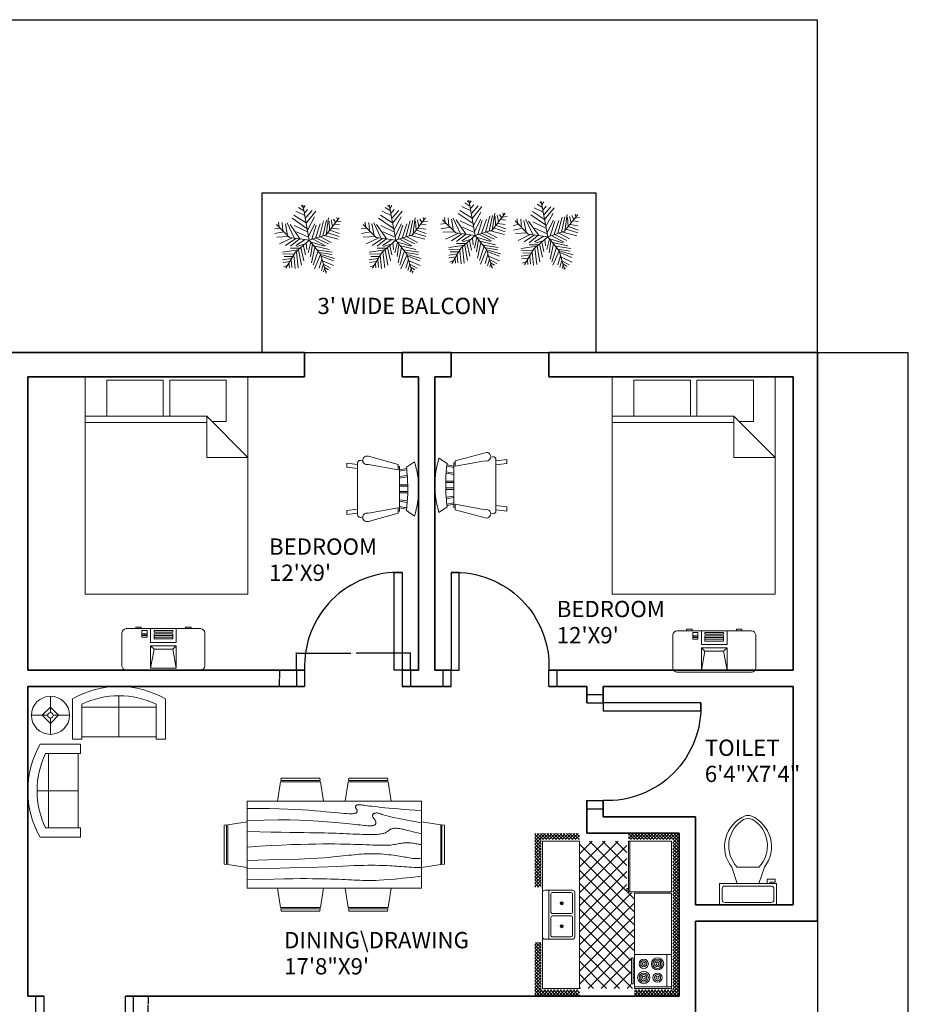
# Model space of a CAD drawing. Units: inches. Extents: x 4159 to 4826, y 299 to 1026.
# Tile 37 of 37: x 4498 to 4826, y 663 to 1026. Entities that reach past the tile are written whole.
import ezdxf

# ---------------------------------------------------------------- set-up
doc = ezdxf.new("R2010")
doc.units = ezdxf.units.IN
for name, color, linetype, lineweight in [('A-ANNO-DIMS', 2, 'Continuous', 18), ('A-AREA-IDEN', 7, 'Continuous', 18), ('A-DOOR', 4, 'Continuous', 25), ('A-EQPM', 8, 'Continuous', 13), ('A-FLOR-BALC', 7, 'Continuous', 25), ('A-FLOR-FIXT', 9, 'Continuous', 18), ('A-FURN', 8, 'Continuous', 18), ('A-WALL', 7, 'Continuous', 35), ('L-PLNT', 94, 'Continuous', 13)]:
    doc.layers.add(name, color=color, linetype=linetype, lineweight=lineweight)
doc.styles.get("Standard").update_dxf_attribs({"font": 'arial.ttf'})
doc.dimstyles.get("Standard").update_dxf_attribs({"dimtxt": 0.18, "dimasz": 0.18, "dimexe": 0.18, "dimexo": 0.0625, "dimgap": 0.09, "dimtad": 0, "dimtih": 1, "dimtoh": 1, "dimdec": 4, "dimzin": 0, "dimdsep": 46, "dimtxsty": 'Standard', "dimcen": 0.09, "dimadec": 0, "dimazin": 0, "dimtfac": 1, "dimtdec": 4, "dimtofl": 0, "dimtmove": 0, "dimatfit": 3, "dimfxl": 1, "dimtolj": 1, "dimtzin": 0, "dimarcsym": 0})

# ---------------------------------------------------------------- blocks, each defined once
blk = doc.blocks.new('Lamp - Table')
for p, q in [((0, 7), (0, 1)), ((-1, 0), (-7, 0)), ((0, 3), (-3, 0)), ((-3, 0), (0, -3)), ((3, 0), (0, 3)), ((0, -3), (3, 0)), ((1, 0), (7, 0)), ((0, -1), (0, -7))]:
    blk.add_line(p, q)
for radius in [7, 1]:
    blk.add_circle((0, 0), radius)
blk = doc.blocks.new('Bed - Queen')
for p, q in [((0, -80.00003), (0, 0)), ((0, 0), (59.99999, 0)), ((59.99999, 0), (59.99999, -80.00003)), ((7.99999, -1.2), (28.79998, -1.2)), ((7.99999, -14.4), (7.99999, -1.2)), ((28.79998, -1.2), (28.79998, -14.4)), ((31.19999, -1.2), (51.99999, -1.2)), ((31.19999, -14.4), (31.19999, -1.2)), ((51.99999, -1.2), (51.99999, -16.4)), ((0, -14.4), (44.8, -14.4)), ((59.99999, -29.6), (44.8, -14.4)), ((44.8, -14.4), (44.8, -29.6)), ((44.8, -16.8), (0, -16.8)), ((51.99999, -16.4), (46.79936, -16.4)), ((44.8, -29.6), (59.99999, -29.6)), ((59.99999, -80.00003), (0, -80.00003))]:
    blk.add_line(p, q)
blk = doc.blocks.new('Chair - Rocking')
for p, q in [((-8, -4.5), (-10, -1.5)), ((8, -4.5), (10, -1.5)), ((-8.23428, -6.99939), (-8.3093, -7.47958)), ((-8.23041, -7), (8.23915, -7)), ((-7.5, -4.5), (-7, -7)), ((-6.5, -7), (-7.02225, -4.43)), ((-4.5, -7), (-4.96674, -4.19951)), ((-4, -7), (-4.40532, -4.16272)), ((-1.5, -4.05012), (-1.5, -7)), ((-1, -7), (-1, -4.05012)), ((1, -7), (1, -4.04655)), ((1.5, -4.05012), (1.5, -7)), ((4, -7), (4.40187, -4.18694)), ((4.5, -7), (4.96761, -4.19437)), ((6.5, -7), (7, -4.4057)), ((7.5, -4.5), (7, -7)), ((8.31071, -7.48854), (8.23449, -7.00073)), ((-9, -7.5), (-12, -18.49999)), ((-7, -7.5), (-9, -7.5)), ((-9, -18.49999), (-7, -7.5)), ((7, -7.5), (9, -7.5)), ((9, -18.49999), (7, -7.5)), ((9, -7.5), (12, -18.49999)), ((-10.36644, -20.64523), (-10.5, -21.49999)), ((10.5, -21.49999), (10.3575, -20.58798)), ((-9, -22.49999), (-9.5, -26.49999)), ((0, -22.49999), (-9.5, -22.49999)), ((-8, -26.49999), (-7.5, -22.49999)), ((0, -22.49999), (9.5, -22.49999)), ((8, -26.49999), (7.5, -22.49999)), ((9, -22.49999), (9.5, -26.49999)), ((-9.5, -26.49999), (-8, -26.49999)), ((9.5, -26.49999), (8, -26.49999))]:
    blk.add_line(p, q)
for centre, radius, start, end in [((0, -34.08333), 34.08333, 72.93847, 107.0615), ((0, -68.25004), 64.25, 93.92211, 97.15267), ((0, -68.25004), 64.25, 82.84733, 93.92211), ((-10.5, -18.99999), 1.58114, 161.5651, 18.43495), ((-9.5, -21.49999), 1, 180, 270), ((10.5, -18.99999), 1.58114, 161.5651, 18.43495), ((9.5, -21.49999), 1, 270, 0)]:
    blk.add_arc(centre, radius, start, end)
blk = doc.blocks.new('Sofa - Roundback Loveseat 5 ft.')
for p, q in [((0, -32.44198), (0, -5.99998)), ((-24, -33.99998), (-24, -11.46958)), ((24.00004, -33.99998), (24.00004, -11.46958)), ((-23.9998, -13.38178), (23.99986, -13.38178)), ((-24, -32.44198), (24.00004, -32.44198))]:
    blk.add_line(p, q)
for points in [[(-24, -33.99998), (-30, -33.99998), (-30, -7.99998)], [(30.00004, -7.99998), (30.00004, -33.99998), (24.00004, -33.99998)]]:
    blk.add_lwpolyline(points)
for centre, radius, start, end in [((0, -60.24998), 60.24998, 60.13715, 119.8628), ((0, -61.38438), 55.38444, 64.32083, 115.6792)]:
    blk.add_arc(centre, radius, start, end)
blk = doc.blocks.new('Dining Set - 36 x 72 in.')
for p, q in [((-22.2343, 26.00059), (-23.4847, 17.99762)), ((-22.2304, 26), (-5.7608, 26)), ((-22, 27.5), (-22.1562, 26.50042)), ((-5.8416, 26.5), (-22.1534, 26.5)), ((-22, 27.5), (-6, 27.5)), ((-5.8437, 26.49966), (-6, 27.5)), ((-4.5152, 17.99762), (-5.7655, 25.99926)), ((5.7657, 26.00059), (4.5153, 17.99762)), ((5.7696, 26), (22.2392, 26)), ((6, 27.5), (5.8438, 26.50042)), ((22.1584, 26.5), (5.8466, 26.5)), ((6, 27.5), (22, 27.5)), ((22.1563, 26.49966), (22, 27.5)), ((23.4848, 17.99762), (22.2345, 25.99926)), ((36, 18), (-36, 18)), ((-36, 18), (-36, -18)), ((36, -18), (36, 18)), ((-45.5, 8), (-44.5004, 8.15617)), ((-44.5, -8.15843), (-44.5, 8.15338)), ((-44.0006, 8.23428), (-35.9976, 9.48474)), ((-44, 8.23041), (-44, -8.23915)), ((44.0006, 8.23428), (35.9976, 9.48474)), ((44, 8.23041), (44, -8.23915)), ((44.5, -8.15843), (44.5, 8.15338)), ((45.5, 8), (44.5005, 8.15617)), ((-45.5, 8), (-45.5, -8)), ((45.5, 8), (45.5, -8)), ((-44.4997, -8.15631), (-45.5, -8)), ((44.4997, -8.15631), (45.5, -8)), ((-35.9976, -9.48476), (-43.9993, -8.2345)), ((35.9976, -9.48476), (43.9993, -8.2345)), ((-36, -18), (36, -18)), ((-22.2343, -26.0006), (-23.4847, -17.99762)), ((-4.5152, -17.99762), (-5.7655, -25.99928)), ((5.7657, -26.0006), (4.5153, -17.99762)), ((23.4848, -17.99762), (22.2345, -25.99928)), ((-22.2304, -26), (-5.7608, -26)), ((-22, -27.5), (-22.1562, -26.50044)), ((-5.8416, -26.5), (-22.1534, -26.5)), ((-22, -27.5), (-6, -27.5)), ((-5.8437, -26.49967), (-6, -27.5)), ((5.7696, -26), (22.2392, -26)), ((6, -27.5), (5.8438, -26.50044)), ((22.1584, -26.5), (5.8466, -26.5)), ((6, -27.5), (22, -27.5)), ((22.1563, -26.49967), (22, -27.5))]:
    blk.add_line(p, q)
for points in [[(-36, 15), (-31.1772, 14.97754), (-26.8079, 14.91406), (-22.8538, 14.81543), (-19.276, 14.6875), (-16.0362, 14.53613), (-13.0957, 14.36718), (-10.4159, 14.18652), (-7.9583, 14), (-5.6904, 13.81315), (-3.6035, 13.63021), (-1.6954, 13.45508), (0.0365, 13.29166), (1.5945, 13.14388), (2.9811, 13.01562), (4.1988, 12.9108), (5.25, 12.83333), (6.1393, 12.78613), (6.8802, 12.76823), (7.4883, 12.77767), (7.9792, 12.8125), (8.3685, 12.87077), (8.6719, 12.95052), (8.9049, 13.0498), (9.0833, 13.16666), (9.2205, 13.29899), (9.3216, 13.44401), (9.3895, 13.59879), (9.4271, 13.76041), (9.4373, 13.92594), (9.4232, 14.09245), (9.3875, 14.257), (9.3333, 14.41666), (9.2638, 14.56917), (9.1836, 14.71484), (9.0975, 14.85465), (9.0104, 14.98958), (8.9272, 15.1206), (8.8529, 15.2487), (8.7922, 15.37483), (8.75, 15.5), (8.7305, 15.62467), (8.7344, 15.74739), (8.7617, 15.86621), (8.8125, 15.97916), (8.8867, 16.08431), (8.9844, 16.17968), (9.1055, 16.26334), (9.25, 16.33333), (9.4189, 16.38802), (9.6172, 16.42708), (9.8506, 16.45052), (10.125, 16.45833), (10.4463, 16.45052), (10.8203, 16.42708), (11.2529, 16.38802), (11.75, 16.33333), (12.3184, 16.26318), (12.9694, 16.17838), (13.7151, 16.07991), (14.5677, 15.96875), (15.5395, 15.84586), (16.6426, 15.71224), (17.8893, 15.56884), (19.2917, 15.41666), (20.859, 15.25667), (22.5879, 15.08984), (24.4721, 14.91715), (26.5052, 14.73958), (28.6809, 14.5581), (30.9929, 14.3737), (33.4347, 14.18733), (36, 14)], [(-36, 10), (-28.9766, 10.14274), (-23.1725, 10.20442), (-18.4241, 10.19775), (-14.5677, 10.13541), (-11.4399, 10.03011), (-8.877, 9.89453), (-6.7154, 9.74137), (-4.7917, 9.58333), (-2.9698, 9.43082), (-1.2246, 9.28515), (0.4415, 9.14534), (2.026, 9.01041), (3.5266, 8.87939), (4.9408, 8.7513), (6.266, 8.62516), (7.5, 8.5), (8.6411, 8.37549), (9.6914, 8.2539), (10.6538, 8.13818), (11.5312, 8.03125), (12.3267, 7.93603), (13.043, 7.85547), (13.6831, 7.79248), (14.25, 7.75), (14.7471, 7.7303), (15.1797, 7.73307), (15.5537, 7.75732), (15.875, 7.80208), (16.1494, 7.86637), (16.3828, 7.94922), (16.5811, 8.04964), (16.75, 8.16666), (16.8944, 8.29915), (17.0143, 8.44531), (17.1089, 8.60319), (17.1771, 8.77083), (17.218, 8.94629), (17.2305, 9.1276), (17.2137, 9.31282), (17.1667, 9.5), (17.0895, 9.6875), (16.987, 9.875), (16.8649, 10.0625), (16.7292, 10.25), (16.5856, 10.4375), (16.4401, 10.625), (16.2985, 10.8125), (16.1667, 11), (16.05, 11.18733), (15.9518, 11.3737), (15.8752, 11.5581), (15.8229, 11.73958), (15.798, 11.91715), (15.8034, 12.08984), (15.842, 12.25667), (15.9167, 12.41666), (16.0295, 12.56836), (16.1784, 12.70833), (16.3605, 12.83268), (16.5729, 12.9375), (16.8127, 13.01888), (17.0768, 13.07291), (17.3625, 13.0957), (17.6667, 13.08333), (17.9894, 13.03312), (18.3418, 12.94726), (18.7382, 12.82918), (19.1927, 12.68229), (19.7195, 12.51001), (20.3327, 12.31575), (21.0465, 12.10294), (21.875, 11.875), (22.8357, 11.63354), (23.959, 11.37304), (25.2786, 11.08618), (26.8282, 10.76562), (28.6414, 10.40405), (30.752, 9.99414), (33.1936, 9.52856), (36, 9)], [(-36, 5.5), (-30.7157, 5.3348), (-26.069, 5.20963), (-21.9946, 5.11767), (-18.4271, 5.05208), (-15.3009, 5.00602), (-12.5508, 4.97265), (-10.1112, 4.94515), (-7.9167, 4.91666), (-5.909, 4.88167), (-4.0586, 4.83984), (-2.3429, 4.79215), (-0.7396, 4.73958), (0.7739, 4.6831), (2.22, 4.6237), (3.6213, 4.56233), (5, 4.5), (6.373, 4.43782), (7.7344, 4.3776), (9.0723, 4.32129), (10.375, 4.27083), (11.6309, 4.22819), (12.8281, 4.19531), (13.9551, 4.17415), (15, 4.16666), (15.954, 4.17448), (16.819, 4.19791), (17.6001, 4.23698), (18.3021, 4.29166), (18.9299, 4.36198), (19.4883, 4.44791), (19.9823, 4.54948), (20.4167, 4.66666), (20.7969, 4.79899), (21.1302, 4.94401), (21.4245, 5.09879), (21.6875, 5.26041), (21.9271, 5.42594), (22.1511, 5.59245), (22.3672, 5.757), (22.5834, 5.91666), (22.8065, 6.06868), (23.0404, 6.21093), (23.2879, 6.34147), (23.5521, 6.45833), (23.8358, 6.55957), (24.142, 6.64323), (24.4735, 6.70735), (24.8334, 6.75), (25.2235, 6.76969), (25.642, 6.76692), (26.0858, 6.74267), (26.5521, 6.69791), (27.0379, 6.63362), (27.5404, 6.55078), (28.0565, 6.45036), (28.5834, 6.33333), (29.1242, 6.19987), (29.7071, 6.04687), (30.3661, 5.87044), (31.1354, 5.66666), (32.0493, 5.43164), (33.142, 5.16146), (34.4475, 4.85221), (36, 4.5)], [(-36, -1), (-30.7915, -0.6591), (-26.0195, -0.38216), (-21.6519, -0.16284), (-17.6563, 0.00521), (-14.0005, 0.12833), (-10.6523, 0.21289), (-7.5796, 0.26522), (-4.75, 0.29166), (-2.134, 0.29793), (0.2878, 0.28711), (2.5317, 0.26163), (4.6146, 0.22396), (6.5529, 0.17651), (8.3633, 0.12174), (10.0623, 0.06209), (11.6667, 0), (13.1899, -0.06201), (14.6341, -0.1211), (15.9982, -0.17432), (17.2813, -0.21875), (18.4823, -0.25147), (19.6003, -0.26953), (20.6343, -0.27002), (21.5834, -0.25), (22.4481, -0.20768), (23.2357, -0.14584), (23.9549, -0.06836), (24.6146, 0.02083), (25.2235, 0.11784), (25.7904, 0.21875), (26.3241, 0.31966), (26.8334, 0.41666), (27.3265, 0.50618), (27.8099, 0.58593), (28.2894, 0.65397), (28.7709, 0.70833), (29.2601, 0.74707), (29.763, 0.76823), (30.2855, 0.76985), (30.8334, 0.75), (31.4088, 0.70784), (31.9994, 0.64713), (32.589, 0.57275), (33.1615, 0.48958), (33.7008, 0.4025), (34.1908, 0.3164), (34.6153, 0.23616), (34.9584, 0.16666), (35.2099, 0.11165), (35.3848, 0.07031), (35.504, 0.04069), (35.5886, 0.02083), (35.6594, 0.00879), (35.7377, 0.0026), (35.8442, 0.00032), (36, 0)], [(-36, -6.5), (-27.1843, -6.31267), (-20.084, -6.1263), (-14.469, -5.9419), (-10.1094, -5.76042), (-6.7752, -5.58285), (-4.2363, -5.41016), (-2.2629, -5.24333), (-0.625, -5.08334), (0.8708, -4.93099), (2.2715, -4.78646), (3.5872, -4.64974), (4.8281, -4.52084), (6.0046, -4.39974), (7.127, -4.28646), (8.2053, -4.18099), (9.25, -4.08334), (10.2705, -3.99382), (11.2734, -3.91407), (12.2647, -3.84603), (13.25, -3.79167), (14.2354, -3.75293), (15.2266, -3.73177), (16.2295, -3.73015), (17.25, -3.75), (18.2912, -3.79248), (19.3451, -3.85547), (20.4009, -3.93604), (21.4479, -4.03125), (22.4754, -4.13819), (23.4727, -4.25391), (24.4289, -4.37549), (25.3334, -4.5), (26.1785, -4.62492), (26.9694, -4.74935), (27.7145, -4.87281), (28.4219, -4.99479), (29.1, -5.11483), (29.7572, -5.23242), (30.4016, -5.34709), (31.0417, -5.45834), (31.6837, -5.56437), (32.3262, -5.65821), (32.9658, -5.73153), (33.599, -5.77604), (34.2224, -5.78345), (34.8327, -5.74545), (35.4264, -5.65373), (36, -5.5)], [(-36, -10), (-26.4022, -9.81299), (-18.4675, -9.62891), (-11.9839, -9.45069), (-6.7396, -9.28125), (-2.5226, -9.12354), (0.8789, -8.98047), (3.6769, -8.85498), (6.0833, -8.75), (8.2767, -8.66765), (10.3021, -8.60677), (12.1712, -8.56543), (13.8958, -8.54167), (15.4876, -8.53353), (16.9583, -8.53907), (18.3197, -8.55632), (19.5834, -8.58334), (20.7616, -8.61841), (21.8685, -8.66081), (22.9188, -8.71004), (23.9271, -8.76563), (24.9081, -8.82707), (25.8763, -8.89388), (26.8465, -8.96558), (27.8334, -9.04167), (28.8474, -9.12118), (29.8828, -9.20117), (30.93, -9.27824), (31.9792, -9.34896), (33.0205, -9.40991), (34.0443, -9.45768), (35.0407, -9.48885), (36, -9.5)], [(-36, -14.5), (-30.0881, -14.33513), (-25.0332, -14.21224), (-20.7312, -14.12647), (-17.0781, -14.07292), (-13.97, -14.04671), (-11.3027, -14.04297), (-8.9724, -14.05681), (-6.875, -14.08334), (-4.9224, -14.11833), (-3.0905, -14.16016), (-1.3709, -14.20785), (0.2448, -14.26042), (1.7647, -14.3169), (3.1973, -14.3763), (4.5507, -14.43767), (5.8333, -14.5), (7.0554, -14.5621), (8.235, -14.62175), (9.3922, -14.67652), (10.5469, -14.72396), (11.7192, -14.76164), (12.929, -14.78711), (14.1965, -14.79794), (15.5417, -14.79167), (16.9933, -14.76424), (18.6152, -14.70508), (20.4804, -14.60197), (22.6615, -14.44271), (25.2312, -14.21509), (28.2624, -13.9069), (31.8277, -13.50594), (36, -13)]]:
    blk.add_lwpolyline(points)
blk = doc.blocks.new('Toilet - top')
for p, q in [((9.5, -6), (9.5, -2)), ((-10, -8.5), (-8, -8.5)), ((-10, -9.5), (-10, -8.5)), ((-7, -9.5), (-10, -9.5)), ((-8, -8.5), (-8, -8)), ((-7, -8), (-7, -9.5)), ((-4, -8), (-6, -14)), ((4, -8), (6, -14)), ((4, -14), (-4, -14))]:
    blk.add_line(p, q)
blk.add_lwpolyline([(10.5, -8), (10.5, 0), (-10.5, 0), (-10.5, -8)], close=True)
for points in [[(-9.5, -2), (-9.5, -6)], [(8.5, -1), (-8.5, -1)], [(-8.5, -7), (8.5, -7)]]:
    blk.add_lwpolyline(points)
for centre, radius, start, end in [((-8.62, -1.88), 0.884, 81.8699, 188.1301), ((8.62, -1.88), 0.884, 351.8699, 98.1301), ((-8.62, -6.12), 0.884, 171.8699, 278.1301), ((8.62, -6.12), 0.884, 261.8699, 8.1301), ((3.52, -21.58), 12.17, 141.4691, 247.9714), ((4.2, -21.82), 11.33, 136.3677, 238.9468), ((-3.52, -21.58), 12.17, 292.0284, 38.5307), ((-4.2, -21.82), 11.33, 301.053, 43.6321), ((0, -27.88), 4, 245.7318, 294.2682), ((0, -29), 4, 254.8605, 285.1395)]:
    blk.add_arc(centre, radius, start, end)
blk = doc.blocks.new('Desk - 30 x 60 in.')
for p, q in [((-26.999995, 0), (26.999995, 0)), ((-29.999995, -27), (-29.999995, -3)), ((29.999995, -3), (29.999995, -27)), ((26.999995, -30), (-26.999995, -30)), ((-20.000005, -30), (-20.000005, -31)), ((-20.000005, -31), (-16.000005, -31)), ((-16.000005, -31), (-16.000005, -30)), ((15.999995, -31), (15.999995, -30)), ((19.999995, -31), (15.999995, -31)), ((19.999995, -30), (19.999995, -31))]:
    blk.add_line(p, q)
for centre, start, end in [((-26.499995, -3.5), 98.1301, 171.8699), ((26.499995, -3.5), 8.130102, 81.8699), ((-26.499995, -26.5), 188.1301, 261.8699), ((26.499995, -26.5), 278.1301, 351.8699)]:
    blk.add_arc(centre, 3.535534, start, end)
blk = doc.blocks.new('Computer Terminal')
for p, q in [((-10, 11.5), (5, 11.5)), ((-8, 0.5), (-10, 11.5)), ((-10, -1.5), (-10, 11.5)), ((5, 11.5), (3, 0.5)), ((5, 11.5), (5, -1.5)), ((-10, -1.5), (-8, 0.5)), ((3, 0.5), (-8, 0.5)), ((3, 0.5), (5, -1.5)), ((5, -1.5), (-10, -1.5)), ((-10, -11.5), (-10, -3.5)), ((-10, -3.5), (5, -3.5)), ((-8, -5.5), (-8, -8.5)), ((3, -5.5), (-8, -5.5)), ((3, -8.5), (3, -5.5)), ((5, -3.5), (5, -11.5)), ((3, -6.5), (-8, -6.5)), ((-8, -7.5), (3, -7.5)), ((-8, -8.5), (3, -8.5)), ((-8, -9.5), (-8, -10.5)), ((3, -9.5), (-8, -9.5)), ((-8, -10.5), (3, -10.5)), ((3, -10.5), (3, -9.5)), ((10, -6.5), (7, -6.5)), ((7, -6.5), (7, -10.5)), ((7, -10.5), (10, -10.5)), ((9.5, -7.5), (7.5, -7.5)), ((7.5, -7.5), (7.5, -8.5)), ((7.5, -8.5), (9.5, -8.5)), ((8.5, -7.5), (8.5, -8.5)), ((9.5, -8.5), (9.5, -7.5)), ((10, -10.5), (10, -6.5)), ((5, -11.5), (-10, -11.5))]:
    blk.add_line(p, q)
blk = doc.blocks.new('Kitchen Layout - 7 x 8 ft')
for p, q in [((-5, 81.32), (2.68, 89)), ((-5, 83.44), (0.56, 89)), ((-5, 85.56), (-1.56, 89)), ((-5, 87.68), (-3.68, 89)), ((-1, 84.97), (-5, 88.97)), ((-1, 82.85), (-5, 86.85)), ((-1, 80.73), (-5, 84.73)), ((1.09, 85), (-2.91, 89)), ((3.21, 85), (-0.79, 89)), ((0.81, 85), (4.81, 89)), ((5.34, 85), (1.34, 89)), ((2.93, 85), (6.93, 89)), ((7.46, 85), (3.46, 89)), ((5.05, 85), (9.05, 89)), ((9.58, 85), (5.58, 89)), ((7.17, 85), (11.17, 89)), ((11.7, 85), (7.7, 89)), ((9.29, 85), (13.29, 89)), ((13.82, 85), (9.82, 89)), ((11.41, 85), (15.41, 89)), ((15.94, 85), (11.94, 89)), ((13.53, 85), (17.53, 89)), ((18.06, 85), (14.06, 89)), ((15.65, 85), (19.65, 89)), ((20.18, 85), (16.18, 89)), ((17.78, 85), (21.78, 89)), ((22.31, 85), (18.31, 89)), ((19.9, 85), (23.9, 89)), ((24.43, 85), (20.43, 89)), ((22.02, 85), (26.02, 89)), ((26.55, 85), (22.55, 89)), ((24.14, 85), (28.14, 89)), ((28.67, 85), (24.67, 89)), ((26.26, 85), (30.26, 89)), ((30.79, 85), (26.79, 89)), ((28.38, 85), (32.38, 89)), ((32.91, 85), (28.91, 89)), ((30.5, 85), (34.5, 89)), ((35.03, 85), (31.03, 89)), ((32.63, 85), (36.63, 89)), ((37.16, 85), (33.16, 89)), ((34, 84), (96, 84)), ((34, 60), (34, 84)), ((34.75, 85), (38.75, 89)), ((39.28, 85), (35.28, 89)), ((36.87, 85), (40.87, 89)), ((41.4, 85), (37.4, 89)), ((38.99, 85), (42.99, 89)), ((43.52, 85), (39.52, 89)), ((41.11, 85), (45.11, 89)), ((45.64, 85), (41.64, 89)), ((43.23, 85), (47.23, 89)), ((47.76, 85), (43.76, 89)), ((45.35, 85), (49.35, 89)), ((49.88, 85), (45.88, 89)), ((47.47, 85), (51.47, 89)), ((52, 85), (48, 89)), ((49.6, 85), (53.6, 89)), ((54.13, 85), (50.13, 89)), ((51.72, 85), (55.72, 89)), ((56.25, 85), (52.25, 89)), ((53.84, 85), (57.84, 89)), ((58.37, 85), (54.37, 89)), ((55.96, 85), (59.96, 89)), ((60.49, 85), (56.49, 89)), ((58.08, 85), (62.08, 89)), ((62.61, 85), (58.61, 89)), ((60.2, 85), (64.2, 89)), ((64.73, 85), (60.73, 89)), ((62.32, 85), (66.32, 89)), ((66.85, 85), (62.85, 89)), ((64.45, 85), (68.45, 89)), ((68.97, 85), (64.97, 89)), ((66.57, 85), (70.57, 89)), ((71.1, 85), (67.1, 89)), ((68.69, 85), (72.69, 89)), ((73.22, 85), (69.22, 89)), ((70.81, 85), (74.81, 89)), ((75.34, 85), (71.34, 89)), ((72.93, 85), (76.93, 89)), ((77.46, 85), (73.46, 89)), ((75.05, 85), (79.05, 89)), ((79.58, 85), (75.58, 89)), ((77.17, 85), (81.17, 89)), ((81.7, 85), (77.7, 89)), ((79.29, 85), (83.29, 89)), ((83.82, 85), (79.82, 89)), ((81.42, 85), (85.42, 89)), ((85.95, 85), (81.95, 89)), ((83.54, 85), (87.54, 89)), ((88.07, 85), (84.07, 89)), ((85.66, 85), (89.66, 89)), ((90.19, 85), (86.19, 89)), ((87.78, 85), (91.78, 89)), ((92.31, 85), (88.31, 89)), ((89.9, 85), (93.9, 89)), ((94.43, 85), (90.43, 89)), ((92.02, 85), (96.02, 89)), ((96.55, 85), (92.55, 89)), ((94.14, 85), (98.14, 89)), ((101, 82.67), (94.67, 89)), ((96, 84), (96, 60)), ((96.27, 85), (100.27, 89)), ((101, 84.79), (96.79, 89)), ((97, 83.61), (101, 87.61)), ((97, 81.49), (101, 85.49)), ((101, 80.55), (97, 84.55)), ((101, 86.92), (98.92, 89)), ((-5, 79.19), (-1, 83.19)), ((-1, 78.61), (-5, 82.61)), ((-5, 77.07), (-1, 81.07)), ((-1, 76.49), (-5, 80.49)), ((-5, 74.95), (-1, 78.95)), ((-1, 74.36), (-5, 78.36)), ((74, 81), (95, 81)), ((97, 79.37), (101, 83.37)), ((101, 78.43), (97, 82.43)), ((97, 77.25), (101, 81.25)), ((101, 76.31), (97, 80.31)), ((97, 75.13), (101, 79.13)), ((101, 74.19), (97, 78.19)), ((-5, 72.83), (-1, 76.83)), ((-1, 72.24), (-5, 76.24)), ((-5, 70.71), (-1, 74.71)), ((-1, 70.12), (-5, 74.12)), ((-5, 68.59), (-1, 72.59)), ((-1, 68), (-5, 72)), ((97, 73.01), (101, 77.01)), ((101, 72.07), (97, 76.07)), ((97, 70.89), (101, 74.89)), ((101, 69.95), (97, 73.95)), ((97, 68.76), (101, 72.76)), ((101, 67.82), (97, 71.82)), ((97, 66.64), (101, 70.64)), ((-5, 66.47), (-1, 70.47)), ((-1, 65.88), (-5, 69.88)), ((-5, 64.35), (-1, 68.35)), ((-1, 63.76), (-5, 67.76)), ((-5, 62.22), (-1, 66.22)), ((-1, 61.64), (-5, 65.64)), ((101, 65.7), (97, 69.7)), ((97, 64.52), (101, 68.52)), ((101, 63.58), (97, 67.58)), ((97, 62.4), (101, 66.4)), ((101, 61.46), (97, 65.46)), ((97, 60.28), (101, 64.28)), ((-5, 60.1), (-1, 64.1)), ((-1, 59.52), (-5, 63.52)), ((-5, 57.98), (-1, 61.98)), ((-1, 57.39), (-5, 61.39)), ((-1.73, 56), (-5, 59.27)), ((-4.86, 56), (-1, 59.86)), ((10.4, 24), (45.9, 59.5)), ((18.88, 24), (54.38, 59.5)), ((27.37, 24), (62.87, 59.5)), ((33.03, 55.11), (37.41, 59.5)), ((67.71, 24), (33.68, 58.04)), ((96, 60), (34, 60)), ((35.85, 24), (71.35, 59.5)), ((76.2, 24), (40.7, 59.5)), ((84.68, 24), (49.18, 59.5)), ((93.17, 24), (57.67, 59.5)), ((61.31, 24), (96, 58.69)), ((96, 29.65), (66.15, 59.5)), ((80, 60), (80, 59)), ((82, 59), (82, 60)), ((87, 59), (87, 60)), ((89, 60), (89, 59)), ((100.34, 60), (97, 63.34)), ((98.22, 60), (97, 61.22)), ((98.84, 60), (101, 62.16)), ((100.96, 60), (101, 60.04)), ((-3.85, 56), (-5, 57.15)), ((-2.74, 56), (-1, 57.74)), ((0, 57), (33, 57)), ((0, 30.57), (24.43, 55)), ((0, 39.06), (15.94, 55)), ((0, 47.54), (7.46, 55)), ((1.91, 24), (32.91, 55)), ((33.77, 24), (2.77, 55)), ((42.26, 24), (11.26, 55)), ((50.74, 24), (19.74, 55)), ((59.23, 24), (28.23, 55)), ((31, 55), (31, 56)), ((32, 55), (31, 55)), ((32, 56), (32, 55)), ((44.34, 24), (77.84, 57.5)), ((52.82, 24), (86.32, 57.5)), ((96, 38.14), (76.64, 57.5)), ((96, 46.63), (85.13, 57.5)), ((96, 55.11), (93.57, 57.54)), ((25.29, 24), (0, 49.29)), ((69.79, 24), (96, 50.21)), ((16.8, 24), (0, 40.8)), ((78.28, 24), (96, 41.72)), ((8.32, 24), (0, 32.32)), ((86.76, 24), (96, 33.24)), ((-5, 21.92), (-2.92, 24)), ((-5, 19.8), (-1, 23.8)), ((-1, 19.21), (-5, 23.21)), ((-5, 17.68), (-1, 21.68)), ((-1, 17.09), (-5, 21.09)), ((-5, 15.55), (-1, 19.55)), ((-1, 21.33), (-3.67, 24)), ((-1, 23.45), (-1.55, 24)), ((0, 24), (96, 24)), ((0, 0), (0, 24)), ((95.25, 24), (96, 24.75)), ((96, 24), (96, 0)), ((97, 22.1), (98.9, 24)), ((97, 19.97), (101, 23.97)), ((101, 19.03), (97, 23.03)), ((97, 17.85), (101, 21.85)), ((101, 16.91), (97, 20.91)), ((97, 15.73), (101, 19.73)), ((101, 21.16), (98.16, 24)), ((101, 23.28), (100.28, 24)), ((-1, 14.97), (-5, 18.97)), ((-5, 13.43), (-1, 17.43)), ((-1, 12.85), (-5, 16.85)), ((-5, 11.31), (-1, 15.31)), ((-1, 10.73), (-5, 14.73)), ((-5, 9.19), (-1, 13.19)), ((47.25, 6.5), (47.25, 18.5)), ((48.75, 18.5), (48.75, 6.5)), ((101, 14.79), (97, 18.79)), ((97, 13.61), (101, 17.61)), ((101, 12.67), (97, 16.67)), ((97, 11.49), (101, 15.49)), ((101, 10.55), (97, 14.55)), ((97, 9.37), (101, 13.37)), ((-1, 8.6), (-5, 12.6)), ((-5, 7.07), (-1, 11.07)), ((-1, 6.48), (-5, 10.48)), ((-5, 4.95), (-1, 8.95)), ((-1, 4.36), (-5, 8.36)), ((-5, 2.83), (-1, 6.83)), ((101, 8.43), (97, 12.43)), ((97, 7.25), (101, 11.25)), ((101, 6.31), (97, 10.31)), ((97, 5.12), (101, 9.12)), ((101, 4.18), (97, 8.18)), ((97, 3), (101, 7)), ((-1, 2.24), (-5, 6.24)), ((-5, 0.71), (-1, 4.71)), ((-1, 0.12), (-5, 4.12)), ((-5, -1.42), (-1, 2.58)), ((2, -5), (-5, 2)), ((-5, -3.54), (-1, 0.46)), ((96, 0), (0, 0)), ((64, 4), (32, 4)), ((93.24, -5), (101, 2.76)), ((95.36, -5), (101, 0.64)), ((101, 2.06), (97, 6.06)), ((97, 0.88), (101, 4.88)), ((101, -0.06), (97, 3.94)), ((101, -2.18), (97, 1.82)), ((-0.12, -5), (-5, -0.12)), ((-2.25, -5), (-5, -2.25)), ((-4.37, -5), (-5, -4.37)), ((-4.34, -5), (-0.34, -1)), ((-2.22, -5), (1.78, -1)), ((-0.1, -5), (3.9, -1)), ((4.12, -5), (0.12, -1)), ((2.02, -5), (6.02, -1)), ((6.24, -5), (2.24, -1)), ((4.14, -5), (8.14, -1)), ((8.36, -5), (4.36, -1)), ((6.27, -5), (10.27, -1)), ((10.48, -5), (6.48, -1)), ((8.39, -5), (12.39, -1)), ((12.6, -5), (8.6, -1)), ((10.51, -5), (14.51, -1)), ((14.73, -5), (10.73, -1)), ((12.63, -5), (16.63, -1)), ((16.85, -5), (12.85, -1)), ((14.75, -5), (18.75, -1)), ((18.97, -5), (14.97, -1)), ((16.87, -5), (20.87, -1)), ((21.09, -5), (17.09, -1)), ((18.99, -5), (22.99, -1)), ((23.21, -5), (19.21, -1)), ((21.11, -5), (25.11, -1)), ((25.33, -5), (21.33, -1)), ((23.24, -5), (27.24, -1)), ((27.45, -5), (23.45, -1)), ((25.36, -5), (29.36, -1)), ((29.57, -5), (25.57, -1)), ((27.48, -5), (30, -2.48)), ((30, -3.3), (27.7, -1)), ((29.6, -5), (30, -4.6)), ((30, -1.18), (29.82, -1)), ((66, -2.54), (67.54, -1)), ((66, -4.66), (69.66, -1)), ((69.88, -5), (66, -1.12)), ((67.76, -5), (66, -3.24)), ((67.78, -5), (71.78, -1)), ((72, -5), (68, -1)), ((69.9, -5), (73.9, -1)), ((74.12, -5), (70.12, -1)), ((72.03, -5), (76.03, -1)), ((76.24, -5), (72.24, -1)), ((74.15, -5), (78.15, -1)), ((78.36, -5), (74.36, -1)), ((76.27, -5), (80.27, -1)), ((80.49, -5), (76.49, -1)), ((78.39, -5), (82.39, -1)), ((82.61, -5), (78.61, -1)), ((80.51, -5), (84.51, -1)), ((84.73, -5), (80.73, -1)), ((82.63, -5), (86.63, -1)), ((86.85, -5), (82.85, -1)), ((84.75, -5), (88.75, -1)), ((88.97, -5), (84.97, -1)), ((86.88, -5), (90.88, -1)), ((91.09, -5), (87.09, -1)), ((89, -5), (93, -1)), ((93.21, -5), (89.21, -1)), ((91.12, -5), (95.12, -1)), ((95.34, -5), (91.34, -1)), ((97.46, -5), (93.46, -1)), ((99.58, -5), (95.58, -1)), ((101, -4.3), (97, -0.3)), ((97.48, -5), (101, -1.48)), ((99.6, -5), (101, -3.6))]:
    blk.add_line(p, q)
for points in [[(0, 56), (0, 84), (33, 84), (33, 56)], [(74, 60), (74, 84), (95, 84), (95, 60)], [(76, 58), (76, 59), (93, 59), (93, 58)]]:
    blk.add_lwpolyline(points, close=True)
for points in [[(32, 1.5), (32, 19.5)], [(33.5, 21), (62.5, 21)], [(34.5, 19.5), (46.25, 19.5)], [(49.75, 19.5), (61.5, 19.5)], [(64, 19.5), (64, 1.5)], [(33.5, 6.5), (33.5, 18.5)], [(62.5, 18.5), (62.5, 6.5)], [(62.5, 0), (33.5, 0)], [(46.25, 5.5), (34.5, 5.5)], [(61.5, 5.5), (49.75, 5.5)]]:
    blk.add_lwpolyline(points)
for centre, radius in [((80, 75), 4), ((80, 75), 3), ((89, 75), 3), ((80, 75), 2), ((80, 75), 1), ((89, 75), 2), ((89, 75), 1), ((80, 66), 3), ((80, 66), 2), ((80, 66), 1), ((89, 66), 4), ((89, 66), 3), ((89, 66), 2), ((89, 66), 1), ((40.5, 12.5), 1), ((40.5, 12.5), 0.5), ((55.5, 12.5), 1), ((55.5, 12.5), 0.5)]:
    blk.add_circle(centre, radius)
for centre, radius, start, end in [((33.5, 19.5), 1.5, 90, 180), ((34.5, 18.5), 1, 90, 180), ((46.25, 18.5), 1, 0, 90), ((49.75, 18.5), 1, 90, 180), ((61.5, 18.5), 1, 0, 90), ((62.5, 19.5), 1.5, 0, 90), ((34.5, 6.5), 1, 180, 270), ((46.25, 6.5), 1, 270, 0), ((49.75, 6.5), 1, 180, 270), ((61.5, 6.5), 1, 270, 0), ((33.5, 1.5), 1.5, 180, 270), ((62.5, 1.5), 1.5, 270, 0)]:
    blk.add_arc(centre, radius, start, end)
blk = doc.blocks.new('*U12')
for p, q in [((-8.737, 47.138), (-17.069, 52.711)), ((-10.186, 53.64), (-13.084, 55.962)), ((0, 0), (-10.5, 57)), ((-9.099, 51.782), (-6.563, 55.962)), ((-7.65, 43.423), (-2.578, 49.46)), ((-5.839, 35.992), (4.667, 48.067)), ((-3.665, 19.273), (-27.574, 35.527)), ((-5.114, 28.097), (-24.676, 40.636)), ((-7.288, 39.707), (-21.778, 46.673)), ((-5.114, 27.632), (10.463, 46.673)), ((-2.941, 16.486), (8.652, 37.85)), ((22.055, 7.198), (27.489, 32.277)), ((27, 9), (48, 36)), ((27.127, 9.056), (31.112, 35.992)), ((35.096, 32.741), (37.27, 22.524)), ((38.719, 34.134), (41.979, 28.561)), ((44.153, 36.456), (45.239, 32.741)), ((-47.498, 19.737), (-55.83, 18.344)), ((-31.5, 4.5), (-52.5, 25.5)), ((-48.585, 21.131), (-49.309, 29.026)), ((-43.513, 28.561), (-42.427, 15.558)), ((-38.442, 26.239), (-34.819, 7.663)), ((-35.544, 28.097), (-24.314, 3.947)), ((-14.533, 2.09), (-30.834, 25.31)), ((-24.314, 23.917), (-2.941, 13.7)), ((-1.129, 6.734), (9.014, 26.704)), ((3.942, 1.625), (11.187, 24.381)), ((10.101, 3.483), (17.708, 26.239)), ((16.259, 5.805), (23.142, 31.348)), ((31.836, 30.883), (32.561, 16.486)), ((33.285, 16.486), (48.862, 10.913)), ((36.183, 19.737), (48.137, 17.88)), ((40.53, 25.775), (48.862, 24.846)), ((43.791, 29.954), (51.036, 30.883)), ((-40.615, 13.7), (-55.105, 10.913)), ((-33.37, 6.269), (-52.207, 5.34)), ((-28.299, 3.483), (-47.86, -5.805)), ((-21.416, 3.018), (-38.079, -8.128)), ((0, 0), (-31.5, 4.5)), ((-15.982, 2.09), (-30.11, -9.521)), ((0, 0), (-22.5, -19.5)), ((-6.563, 1.161), (-21.416, -8.128)), ((-20.691, 13.7), (-1.129, 4.876)), ((0, 0), (27, 9)), ((0, 0), (18, -22.5)), ((6.478, 1.625), (26.04, -8.592)), ((11.187, 3.483), (30.749, -5.805)), ((18.07, 5.805), (35.096, -3.483)), ((24.229, 7.663), (46.688, 1.625)), ((29.662, 12.307), (48.137, 6.269)), ((-17.431, -15.094), (-42.789, -18.809)), ((-15.257, -12.772), (-30.11, -12.772)), ((-6.563, -5.805), (-19.967, -9.985)), ((-17.069, -15.094), (-12.721, -40.172)), ((-13.446, -11.378), (-8.737, -32.741)), ((-9.461, -8.592), (-6.201, -23.453)), ((-4.752, -3.483), (-3.665, -14.629)), ((2.493, -3.019), (-1.491, -20.202)), ((1.769, -2.555), (24.229, -9.521)), ((5.029, -6.27), (2.131, -25.775)), ((9.014, -11.378), (3.58, -35.992)), ((7.565, -9.056), (32.198, -14.629)), ((12.274, -15.094), (36.907, -18.809)), ((-28.299, -29.026), (-42.789, -31.348)), ((-24.314, -21.596), (-42.427, -22.06)), ((-26.849, -26.24), (-40.253, -25.775)), ((-22.5, -19.5), (-37.5, -45)), ((-29.023, -30.884), (-27.936, -43.887)), ((-25.038, -23.918), (-22.865, -45.281)), ((-20.691, -18.345), (-17.793, -44.352)), ((14.085, -16.951), (6.478, -40.172)), ((18.07, -22.524), (8.289, -45.745)), ((20.244, -30.419), (15.897, -44.816)), ((16.259, -19.738), (36.183, -22.989)), ((18, -22.5), (27, -52.5)), ((18.433, -22.524), (40.53, -29.026)), ((19.157, -25.311), (38.719, -33.206)), ((-30.834, -34.135), (-42.427, -35.528)), ((-34.457, -39.708), (-40.978, -42.494)), ((-32.646, -36.921), (-31.921, -44.352)), ((22.78, -37.85), (19.519, -48.532)), ((21.331, -32.741), (39.081, -40.636)), ((22.78, -38.314), (34.372, -44.816)), ((24.591, -45.745), (23.142, -50.854)), ((24.591, -43.423), (30.749, -47.603)), ((26.764, -49.925), (28.213, -50.854))]:
    blk.add_line(p, q)
blk = doc.blocks.new('DOOR-SWING-36IN')
blk.add_lwpolyline([(0, 0), (-3, 0), (-3, 36), (0, 36)], close=True)
blk.add_arc((-1.5, 1.5), 34.53, 87.5104, 182.4896)
blk = doc.blocks.new('DOOR-FRAME-36IN')
for p, q in [((0, 6), (0, 0)), ((3, 6), (3, 0)), ((39, 6), (39, 0)), ((42, 6), (42, 0))]:
    blk.add_line(p, q)
blk = doc.blocks.new('DOOR-FRAME-30IN')
for p, q in [((0, 6), (0, 0)), ((3, 6), (3, 0)), ((33, 6), (33, 0)), ((36, 6), (36, 0))]:
    blk.add_line(p, q)
blk = doc.blocks.new('*D19')
at = {"layer": 'A-ANNO-DIMS', "color": 0, "lineweight": -2, "transparency": 16777216}
for p, q in [((4600.31, 786.32), (4600.31, 792.73)), ((4600.49, 792.55), (4620.31, 792.55)), ((4642.13, 792.55), (4622.31, 792.55)), ((4642.31, 786.32), (4642.31, 792.73))]:
    blk.add_line(p, q, dxfattribs=at)
at = {"layer": 'A-ANNO-DIMS', "color": 0, "transparency": 16777216}
for points in [[(4600.49, 792.58), (4600.49, 792.52), (4600.31, 792.55)], [(4642.13, 792.58), (4642.13, 792.52), (4642.31, 792.55)]]:
    blk.add_solid(points, dxfattribs=at)
at = {"layer": 'Defpoints', "color": 0, "transparency": 16777216}
for p in [(4642.31, 792.55), (4600.31, 786.25), (4642.31, 786.25)]:
    blk.add_point(p, dxfattribs=at)
at = {"layer": 'A-ANNO-DIMS', "color": 0, "transparency": 16777216, "insert": (4621.31, 792.55), "char_height": 0.18, "attachment_point": 5}
blk.add_mtext('\\A1;FRAME 42 TYP.', dxfattribs=at)
blk = doc.blocks.new('*D20')
at = {"layer": 'A-ANNO-DIMS', "color": 0, "lineweight": -2, "transparency": 16777216}
for p, q in [((4600.25, 786.25), (4593.83, 786.25)), ((4594.01, 786.07), (4594.01, 783.44)), ((4600.25, 780.25), (4593.83, 780.25)), ((4594.01, 780.43), (4594.01, 783.07))]:
    blk.add_line(p, q, dxfattribs=at)
at = {"layer": 'A-ANNO-DIMS', "color": 0, "transparency": 16777216}
for points in [[(4593.98, 786.07), (4594.04, 786.07), (4594.01, 786.25)], [(4593.98, 780.43), (4594.04, 780.43), (4594.01, 780.25)]]:
    blk.add_solid(points, dxfattribs=at)
at = {"layer": 'Defpoints', "color": 0, "transparency": 16777216}
for p in [(4594.01, 786.25), (4600.31, 786.25), (4600.31, 780.25)]:
    blk.add_point(p, dxfattribs=at)
at = {"layer": 'A-ANNO-DIMS', "color": 0, "transparency": 16777216, "insert": (4594.01, 783.25), "char_height": 0.18, "attachment_point": 5}
blk.add_mtext('\\A1;6 TYP.', dxfattribs=at)
blk = doc.blocks.new('*D22')
at = {"layer": 'A-ANNO-DIMS', "color": 0, "lineweight": -2, "transparency": 16777216}
for p, q in [((4540.37, 666.25), (4545.89, 666.25)), ((4545.71, 666.07), (4545.71, 663.44)), ((4540.37, 660.25), (4545.89, 660.25)), ((4545.71, 660.43), (4545.71, 663.07))]:
    blk.add_line(p, q, dxfattribs=at)
at = {"layer": 'A-ANNO-DIMS', "color": 0, "transparency": 16777216}
for points in [[(4545.68, 666.07), (4545.74, 666.07), (4545.71, 666.25)], [(4545.68, 660.43), (4545.74, 660.43), (4545.71, 660.25)]]:
    blk.add_solid(points, dxfattribs=at)
at = {"layer": 'Defpoints', "color": 0, "transparency": 16777216}
for p in [(4540.31, 666.25), (4540.31, 660.25), (4545.71, 660.25)]:
    blk.add_point(p, dxfattribs=at)
at = {"layer": 'A-ANNO-DIMS', "color": 0, "transparency": 16777216, "insert": (4545.71, 663.25), "char_height": 0.18, "attachment_point": 5}
blk.add_mtext('\\A1;6 TYP.', dxfattribs=at)
blk = doc.blocks.new('*D43')
at = {"layer": 'A-ANNO-DIMS', "color": 0, "lineweight": -2, "transparency": 16777216}
for p, q in [((4192.31, 903.32), (4192.31, 1025.84)), ((4192.49, 1025.66), (4492.02, 1025.66)), ((4792.13, 1025.66), (4492.6, 1025.66)), ((4792.31, 903.32), (4792.31, 1025.84))]:
    blk.add_line(p, q, dxfattribs=at)
at = {"layer": 'A-ANNO-DIMS', "color": 0, "transparency": 16777216}
for points in [[(4192.49, 1025.69), (4192.49, 1025.63), (4192.31, 1025.66)], [(4792.13, 1025.69), (4792.13, 1025.63), (4792.31, 1025.66)]]:
    blk.add_solid(points, dxfattribs=at)
at = {"layer": 'Defpoints', "color": 0, "transparency": 16777216}
for p in [(4792.31, 1025.66), (4192.31, 903.25), (4792.31, 903.25)]:
    blk.add_point(p, dxfattribs=at)
at = {"layer": 'A-ANNO-DIMS', "color": 0, "transparency": 16777216, "insert": (4492.31, 1025.66), "char_height": 0.18, "attachment_point": 5}
blk.add_mtext('\\A1;600', dxfattribs=at)
blk = doc.blocks.new('*D45')
at = {"layer": 'A-ANNO-DIMS', "color": 0, "lineweight": -2, "transparency": 16777216}
for p, q in [((4792.37, 903.25), (4825.74, 903.25)), ((4825.56, 903.07), (4825.56, 647.94)), ((4825.56, 392.43), (4825.56, 647.57)), ((4792.37, 392.25), (4825.74, 392.25))]:
    blk.add_line(p, q, dxfattribs=at)
at = {"layer": 'A-ANNO-DIMS', "color": 0, "transparency": 16777216}
for points in [[(4825.53, 903.07), (4825.59, 903.07), (4825.56, 903.25)], [(4825.53, 392.43), (4825.59, 392.43), (4825.56, 392.25)]]:
    blk.add_solid(points, dxfattribs=at)
at = {"layer": 'Defpoints', "color": 0, "transparency": 16777216}
for p in [(4792.31, 903.25), (4792.31, 392.25), (4825.56, 392.25)]:
    blk.add_point(p, dxfattribs=at)
at = {"layer": 'A-ANNO-DIMS', "color": 0, "transparency": 16777216, "insert": (4825.56, 647.75), "char_height": 0.18, "attachment_point": 5}
blk.add_mtext('\\A1;511', dxfattribs=at)
blk = doc.blocks.new('*D49')
at = {"layer": 'A-ANNO-DIMS', "color": 0, "lineweight": -2, "transparency": 16777216}
for p, q in [((4747.31, 693.73), (4747.31, 298.77)), ((4792.31, 693.73), (4792.31, 298.77)), ((4747.49, 298.95), (4769.59, 298.95)), ((4792.13, 298.95), (4770.03, 298.95))]:
    blk.add_line(p, q, dxfattribs=at)
at = {"layer": 'A-ANNO-DIMS', "color": 0, "transparency": 16777216}
for points in [[(4747.49, 298.98), (4747.49, 298.92), (4747.31, 298.95)], [(4792.13, 298.98), (4792.13, 298.92), (4792.31, 298.95)]]:
    blk.add_solid(points, dxfattribs=at)
at = {"layer": 'Defpoints', "color": 0, "transparency": 16777216}
for p in [(4747.31, 693.79), (4792.31, 693.79), (4792.31, 298.95)]:
    blk.add_point(p, dxfattribs=at)
at = {"layer": 'A-ANNO-DIMS', "color": 0, "transparency": 16777216, "insert": (4769.81, 298.95), "char_height": 0.18, "attachment_point": 5}
blk.add_mtext('\\A1;45', dxfattribs=at)

msp = doc.modelspace()

# ---------------------------------------------------------------- linework, layer by layer
at = {"layer": 'A-FLOR-BALC'}
msp.add_lwpolyline([(4587.531, 903.254), (4710.778, 903.254), (4710.778, 961.989), (4587.531, 961.989)], close=True, dxfattribs=at)
at = {"layer": 'A-WALL'}
for p, q in [((4603.31, 894.254), (4603.31, 903.254)), ((4639.31, 894.254), (4639.31, 903.254)), ((4657.31, 894.254), (4657.31, 903.254)), ((4693.31, 894.254), (4693.31, 903.254)), ((4501.31, 894.254), (4501.31, 786.254)), ((4603.31, 894.254), (4501.31, 894.254)), ((4645.31, 894.254), (4639.31, 894.254)), ((4645.31, 894.254), (4645.31, 786.254)), ((4651.31, 894.254), (4651.31, 786.254)), ((4657.31, 894.254), (4651.31, 894.254)), ((4783.31, 894.254), (4693.31, 894.254)), ((4783.31, 786.254), (4783.31, 894.254)), ((4603.31, 786.254), (4501.31, 786.254)), ((4645.31, 786.254), (4639.31, 786.254)), ((4657.31, 786.254), (4651.31, 786.254)), ((4783.31, 786.254), (4693.31, 786.254)), ((4501.31, 780.254), (4501.31, 666.254)), ((4603.31, 780.254), (4501.31, 780.254)), ((4657.31, 780.254), (4639.31, 780.254)), ((4707.31, 780.254), (4693.31, 780.254)), ((4707.31, 774.254), (4707.31, 780.254)), ((4783.31, 780.254), (4713.31, 780.254)), ((4713.31, 774.254), (4713.31, 780.254)), ((4783.31, 699.788), (4783.31, 780.254)), ((4707.31, 732.254), (4707.31, 738.254)), ((4713.31, 732.254), (4713.31, 738.254)), ((4707.31, 732.254), (4707.31, 726.254)), ((4747.31, 732.254), (4713.31, 732.254)), ((4747.31, 699.788), (4747.31, 732.254)), ((4741.31, 726.254), (4707.31, 726.254)), ((4741.31, 666.254), (4741.31, 726.254)), ((4747.31, 699.788), (4783.31, 699.788)), ((4747.31, 693.788), (4792.31, 693.788)), ((4747.31, 638.43), (4747.31, 693.788)), ((4507.31, 666.254), (4501.31, 666.254)), ((4741.31, 666.254), (4537.31, 666.254))]:
    msp.add_line(p, q, dxfattribs=at)
for points in [[(4603.31, 903.254), (4393.31, 903.254)], [(4657.31, 903.254), (4639.31, 903.254)], [(4792.31, 693.788), (4792.31, 903.254), (4693.31, 903.254)]]:
    msp.add_lwpolyline(points, dxfattribs=at)

# ---------------------------------------------------------------- block references
at = {"layer": 'A-DOOR'}
for name, p in [('DOOR-SWING-36IN', (4639.31, 786.254)), ('DOOR-FRAME-36IN', (4600.31, 780.254))]:
    msp.add_blockref(name, p, dxfattribs=at)
at = {"layer": 'A-DOOR', "extrusion": (0, 0, -1), "zscale": -1}
msp.add_blockref('DOOR-SWING-36IN', (-4657.31, 786.254), dxfattribs=at)
at = {"layer": 'A-DOOR'}
for name, p, rotation in [('DOOR-FRAME-36IN', (4696.31, 786.254), 180), ('DOOR-FRAME-36IN', (4713.31, 735.254), 90.00000000000026), ('DOOR-FRAME-30IN', (4540.31, 666.254), 180)]:
    msp.add_blockref(name, p, dxfattribs=dict(at, rotation=rotation))
at = {"layer": 'A-DOOR', "extrusion": (0, 0, -1), "zscale": -1, "rotation": 90.00000000000175}
msp.add_blockref('DOOR-SWING-36IN', (-4713.31, 774.254), dxfattribs=at)
at = {"layer": 'A-EQPM', "xscale": 0.6328414688201627, "yscale": 0.6328414688201627, "zscale": 0.6328414688201627, "rotation": 180}
for p in [(4549.704, 794.286), (4752.658, 793.532)]:
    msp.add_blockref('Computer Terminal', p, dxfattribs=at)
at = {"layer": 'A-FLOR-FIXT', "rotation": 180}
msp.add_blockref('Toilet - top', (4766.714, 699.739), dxfattribs=at)
at = {"layer": 'A-FLOR-FIXT', "xscale": 0.5650329326971529, "yscale": 0.5650329326971529, "zscale": 0.5650329326971529, "rotation": 270}
msp.add_blockref('Kitchen Layout - 7 x 8 ft', (4690.982, 723.322), dxfattribs=at)
at = {"layer": 'A-FURN'}
for p in [(4522.426, 894.254), (4716.675, 894.254)]:
    msp.add_blockref('Bed - Queen', p, dxfattribs=at)
for p, rotation in [((4645.31, 853.048), 270), ((4651.31, 854.374), 90)]:
    msp.add_blockref('Chair - Rocking', p, dxfattribs=dict(at, rotation=rotation))
for name, p, xscale, yscale, zscale, rotation in [('Desk - 30 x 60 in.', (4551.286, 786.267), 0.5098837128326598, 0.5098837128326598, 0.5098837128326598, 180), ('Desk - 30 x 60 in.', (4754.24, 785.513), 0.5098837128326598, 0.5098837128326598, 0.5098837128326598, 180), ('Sofa - Roundback Loveseat 5 ft.', (4501.31, 741.869), 0.5700533147329089, 0.5700533147329089, 0.5700533147329089, 90)]:
    msp.add_blockref(name, p, dxfattribs=dict(at, xscale=xscale, yscale=yscale, zscale=zscale, rotation=rotation))
for name, p, xscale, yscale, zscale in [('Sofa - Roundback Loveseat 5 ft.', (4534.89, 780.254), 0.5700533147329089, 0.5700533147329089, 0.5700533147329089), ('Lamp - Table', (4509.656, 769.652), 1.003057144141322, 1.003057144141322, 1.003057144141322), ('Dining Set - 36 x 72 in.', (4614.242, 722.009), 0.8913588978043845, 0.8913588978043845, 0.8913588978043845)]:
    msp.add_blockref(name, p, dxfattribs=dict(at, xscale=xscale, yscale=yscale, zscale=zscale))
at = {"layer": 'L-PLNT', "xscale": 0.2292012274639507, "yscale": 0.2292012274639507, "zscale": 0.2292012274639507}
for p in [(4605.017, 944.582), (4636.905, 944.582), (4666.209, 946.304), (4692.926, 945.873)]:
    msp.add_blockref('*U12', p, dxfattribs=at)

# ---------------------------------------------------------------- texts
at = {"layer": 'A-AREA-IDEN'}
for s, p in [("3' WIDE BALCONY", (4608.041, 917.42)), ('BEDROOM', (4590.183, 828.788)), ("12'X9'", (4590.183, 819.149)), ('BEDROOM', (4696.23, 805.795)), ("12'X9'", (4696.23, 796.157)), ('TOILET', (4750.777, 754.7)), ('6\'4"X7\'4"', (4750.777, 745.061)), ('DINING\\DRAWING', (4595.778, 683.846)), ('17\'8"X9\'', (4595.778, 674.207))]:
    msp.add_text(s, height=6, dxfattribs=at).set_placement(p)

# ---------------------------------------------------------------- dimensions: what is measured, and where the dimension line sits
at = {"layer": 'A-ANNO-DIMS'}
for base, p1, p2, picture, middle in [((4792.31, 1025.662), (4192.31, 903.254), (4792.31, 903.254), '*D43', (4492.31, 1025.662)), ((4792.31, 298.945), (4747.31, 693.788), (4792.31, 693.788), '*D49', (4769.81, 298.945))]:
    dim = msp.add_linear_dim(base=base, p1=p1, p2=p2, dimstyle='Standard', override={"dimdec": 0, "dimlfac": 1, "dimrnd": 0, "dimzin": 0, "dimdsep": 46, "dimlunit": 2}, dxfattribs=at)
    dim.commit()
    dim.dimension.update_dxf_attribs({"geometry": picture, "text_midpoint": middle})
dim = msp.add_linear_dim(base=(4825.56, 392.254), p1=(4792.31, 903.254), p2=(4792.31, 392.254), angle=90, dimstyle='Standard', override={"dimdec": 0, "dimlfac": 1, "dimrnd": 0, "dimzin": 0, "dimdsep": 46, "dimlunit": 2}, dxfattribs=at)
dim.commit()
dim.dimension.update_dxf_attribs({"geometry": '*D45', "text_midpoint": (4825.56, 647.754)})
dim = msp.add_linear_dim(base=(4642.31, 792.554), p1=(4600.31, 786.254), p2=(4642.31, 786.254), text='FRAME <> TYP.', dimstyle='Standard', override={"dimdec": 0, "dimlfac": 1, "dimrnd": 0, "dimzin": 0, "dimdsep": 46, "dimlunit": 2}, dxfattribs=at)
dim.commit()
dim.dimension.update_dxf_attribs({"geometry": '*D19', "text_midpoint": (4621.31, 792.554)})
for base, p1, p2, angle, picture, middle in [((4594.01, 786.254), (4600.31, 780.254), (4600.31, 786.254), 90, '*D20', (4594.01, 783.254)), ((4545.71, 660.254), (4540.31, 666.254), (4540.31, 660.254), 270, '*D22', (4545.71, 663.254))]:
    dim = msp.add_linear_dim(base=base, p1=p1, p2=p2, angle=angle, text='<> TYP.', dimstyle='Standard', override={"dimdec": 0, "dimlfac": 1, "dimrnd": 0, "dimzin": 0, "dimdsep": 46, "dimlunit": 2}, dxfattribs=at)
    dim.commit()
    dim.dimension.update_dxf_attribs({"geometry": picture, "text_midpoint": middle})

doc.saveas('drawing.dxf')
